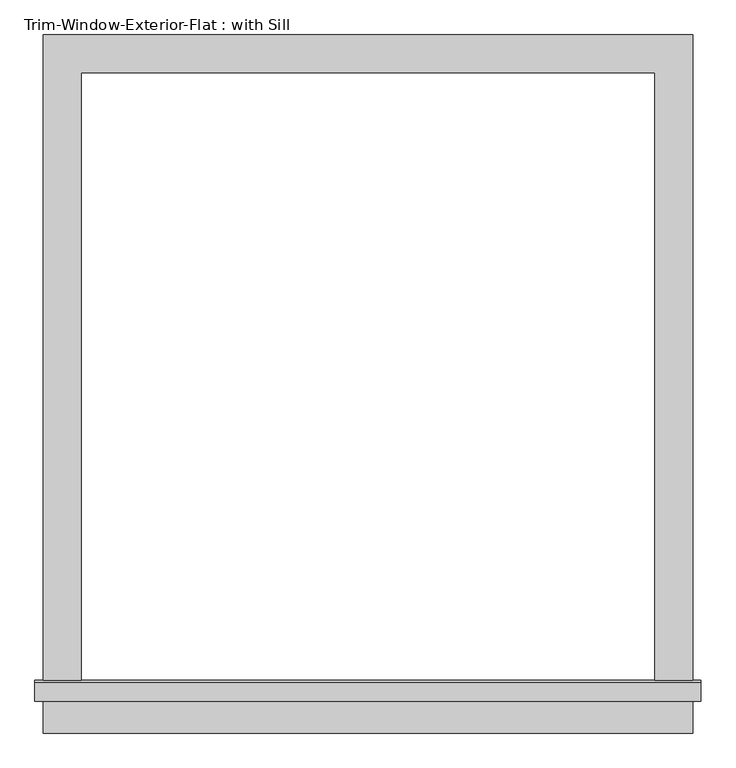
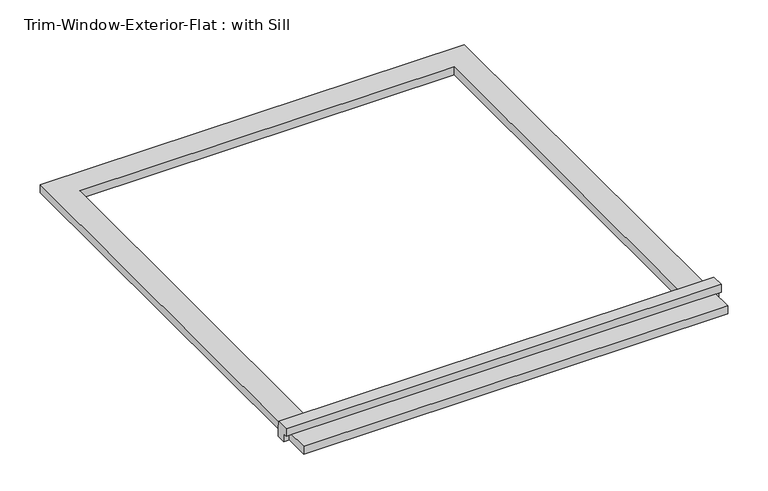
"""IFC4 building model written with IfcOpenShell, lengths in millimetres: proxy geometry, Trim-Window-Exterior-Flat : with Sill."""

from ifc_helpers import new_model, si_unit, frame, origin, origin_with_axes, place, context, project, spatial, polyline, outline, extrude, source, transform, mapped, element, save


def trim_window_exterior_flat_with_sill_41619996(model_context):
    return source(origin(), model_context, "Body", "SweptSolid", [
        extrude(outline(polyline([(488.95, -936.5823709), (488.95, -993.7323709), (-488.95, -993.7323709), (-488.95, -936.5823709), (488.95, -936.5823709)])), origin_with_axes(), (0.0, 0.0, 1.0), 19.05),
        extrude(outline(polyline([(-946.15, 38.1), (-916.8580645, 38.1), (-914.4, 19.05), (-914.4, 0.0), (-936.5823709, 0.0), (-936.5823709, 19.05), (-946.15, 19.05), (-946.15, 38.1)])), frame((-501.65, 0.0, 0.0), z_axis=(1.0, 0.0, 0.0), x_axis=(0.0, 1.0, 0.0)), (0.0, 0.0, 1.0), 1003.3),
        extrude(outline(polyline([(-488.95, 57.15), (488.95, 57.15), (488.95, -914.4), (431.8, -914.4), (431.8, 0.0), (-431.8, 0.0), (-431.8, -914.4), (-488.95, -914.4), (-488.95, 57.15)])), origin_with_axes(), (0.0, 0.0, 1.0), 19.05),
    ])


if __name__ == "__main__":
    model = new_model("IFC4")
    model_context = context("Model", 3, world=origin())
    ifc_project = project(units=[si_unit("LENGTHUNIT", "METRE", prefix="MILLI")], contexts=[model_context])
    site = spatial("IfcSite", under=ifc_project)
    building = spatial("IfcBuilding", under=site)
    placement = place(None, origin())
    trim_window_exterior_flat_with_sill_shape = trim_window_exterior_flat_with_sill_41619996(model_context)
    element("IfcBuildingElementProxy", 1, Name="Trim-Window-Exterior-Flat : with Sill", ObjectType="Trim-Window-Exterior-Flat : with Sill", at=placement, inside=building, context=model_context, shape_type="MappedRepresentation", body=[
        mapped(trim_window_exterior_flat_with_sill_shape, transform((0.0, 0.0, 0.0), x_axis=(1.0, 0.0, 0.0), y_axis=(0.0, 1.0, 0.0), z_axis=(0.0, 0.0, 1.0))),
    ])
    save(model, "model.ifc")

# Revit data of these elements
# Type "Trim-Window-Exterior-Flat : with Sill"
#   Trim Width = 2.25"
#   Trim Thickness_Picture Frame = 1.25"
#   Trim Thickness_with Sill = 0.75"
#   Sill Thickness = 1.25"
#   Opening Width [instance default] = 24"
#   Opening Height [instance default] = 36"
#   Default Elevation = 48"
#   Sill = yes
#   Picture Frame = no
#   Trim Material [instance default] = none
# Element 1 (IfcBuildingElementProxy, "Trim-Window-Exterior-Flat : with Sill")
#   Opening Width = 34"
#   Trim Material = Clad - White
#   Materials on its faces: "Clad - White"
# Materials
#   "Clad - White": class "Wood", colour RGB 242 242 238, transparency 0, Cost = 0
